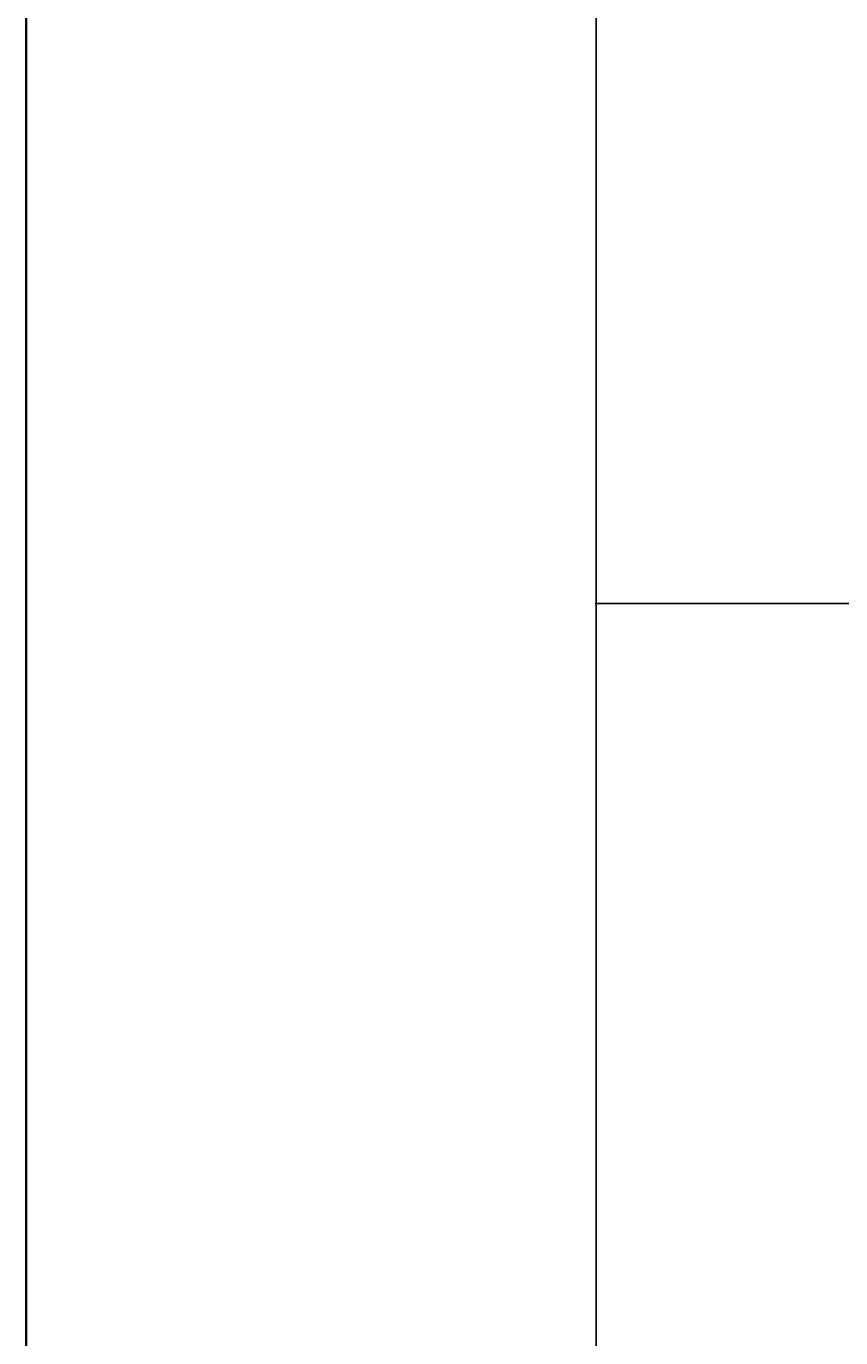
# Model space of a CAD drawing. Units: inches. Extents: x 2120 to 4013, y 1390 to 3019.
# Tile 4 of 59: x 2120 to 2259, y 1740 to 1964. Entities that reach past the tile are written whole.
import ezdxf

# ---------------------------------------------------------------- set-up
doc = ezdxf.new("R2010")
doc.units = ezdxf.units.IN
doc.layers.add('A-ANNO-DIMS', color=2, linetype='Continuous', lineweight=18)
doc.layers.add('A-ANNO-TTLB', color=7, linetype='Continuous', lineweight=35)
doc.styles.get("Standard").update_dxf_attribs({"font": 'arial.ttf'})
doc.dimstyles.get("Standard").update_dxf_attribs({"dimtxt": 0.18, "dimasz": 0.18, "dimexe": 0.18, "dimexo": 0.0625, "dimgap": 0.09, "dimtad": 0, "dimtih": 1, "dimtoh": 1, "dimdec": 4, "dimzin": 0, "dimdsep": 46, "dimtxsty": 'Standard', "dimcen": 0.09, "dimadec": 0, "dimazin": 0, "dimtfac": 1, "dimtdec": 4, "dimtofl": 0, "dimtmove": 0, "dimatfit": 3, "dimfxl": 1, "dimtolj": 1, "dimtzin": 0, "dimarcsym": 0})

# ---------------------------------------------------------------- blocks, each defined once
blk = doc.blocks.new('*D213')
at = {"layer": 'A-ANNO-DIMS', "color": 0, "lineweight": -2, "transparency": 16777216}
for p, q in [((2271.67, 1865.53), (2217.55, 1865.53)), ((2217.73, 1865.35), (2217.73, 1723.71)), ((2217.73, 1581.71), (2217.73, 1723.35)), ((2262.67, 1581.53), (2217.55, 1581.53))]:
    blk.add_line(p, q, dxfattribs=at)
at = {"layer": 'A-ANNO-DIMS', "color": 0, "transparency": 16777216}
for points in [[(2217.7, 1865.35), (2217.76, 1865.35), (2217.73, 1865.53)], [(2217.7, 1581.71), (2217.76, 1581.71), (2217.73, 1581.53)]]:
    blk.add_solid(points, dxfattribs=at)
at = {"layer": 'Defpoints', "color": 0, "transparency": 16777216}
for p in [(2217.73, 1865.53), (2271.73, 1865.53), (2262.73, 1581.53)]:
    blk.add_point(p, dxfattribs=at)
at = {"layer": 'A-ANNO-DIMS', "color": 0, "transparency": 16777216, "insert": (2217.73, 1723.53), "char_height": 0.18, "attachment_point": 5}
blk.add_mtext('\\A1;284', dxfattribs=at)
blk = doc.blocks.new('*D214')
at = {"layer": 'A-ANNO-DIMS', "color": 0, "lineweight": -2, "transparency": 16777216}
for p, q in [((2271.67, 2075.03), (2217.55, 2075.03)), ((2217.73, 2074.85), (2217.73, 1970.46)), ((2217.73, 1865.71), (2217.73, 1970.1)), ((2271.67, 1865.53), (2217.55, 1865.53))]:
    blk.add_line(p, q, dxfattribs=at)
at = {"layer": 'A-ANNO-DIMS', "color": 0, "transparency": 16777216}
for points in [[(2217.7, 2074.85), (2217.76, 2074.85), (2217.73, 2075.03)], [(2217.7, 1865.71), (2217.76, 1865.71), (2217.73, 1865.53)]]:
    blk.add_solid(points, dxfattribs=at)
at = {"layer": 'Defpoints', "color": 0, "transparency": 16777216}
for p in [(2217.73, 2075.03), (2271.73, 2075.03), (2271.73, 1865.53)]:
    blk.add_point(p, dxfattribs=at)
at = {"layer": 'A-ANNO-DIMS', "color": 0, "transparency": 16777216, "insert": (2217.73, 1970.28), "char_height": 0.18, "attachment_point": 5}
blk.add_mtext('\\A1;209.5', dxfattribs=at)

msp = doc.modelspace()

# ---------------------------------------------------------------- linework, layer by layer
at = {"layer": 'A-ANNO-TTLB'}
msp.add_lwpolyline([(2120.4581, 3019.1237), (4012.9334, 3019.1237), (4012.9334, 1390.2222), (2120.4581, 1390.2222)], close=True, dxfattribs=at)

# ---------------------------------------------------------------- dimensions: what is measured, and where the dimension line sits
at = {"layer": 'A-ANNO-DIMS'}
for base, p1, p2, override, picture, middle in [((2217.7331, 2075.031), (2271.7331, 1865.531), (2271.7331, 2075.031), {"dimdec": 1, "dimlfac": 1, "dimrnd": 0, "dimzin": 0, "dimdsep": 46, "dimlunit": 2}, '*D214', (2217.7331, 1970.281)), ((2217.7331, 1865.531), (2262.7331, 1581.531), (2271.7331, 1865.531), {"dimdec": 0, "dimlfac": 1, "dimrnd": 0, "dimzin": 0, "dimdsep": 46, "dimlunit": 2}, '*D213', (2217.7331, 1723.531))]:
    dim = msp.add_linear_dim(base=base, p1=p1, p2=p2, angle=90, dimstyle='Standard', override=override, dxfattribs=at)
    dim.commit()
    dim.dimension.update_dxf_attribs({"geometry": picture, "text_midpoint": middle})

doc.saveas('drawing.dxf')
